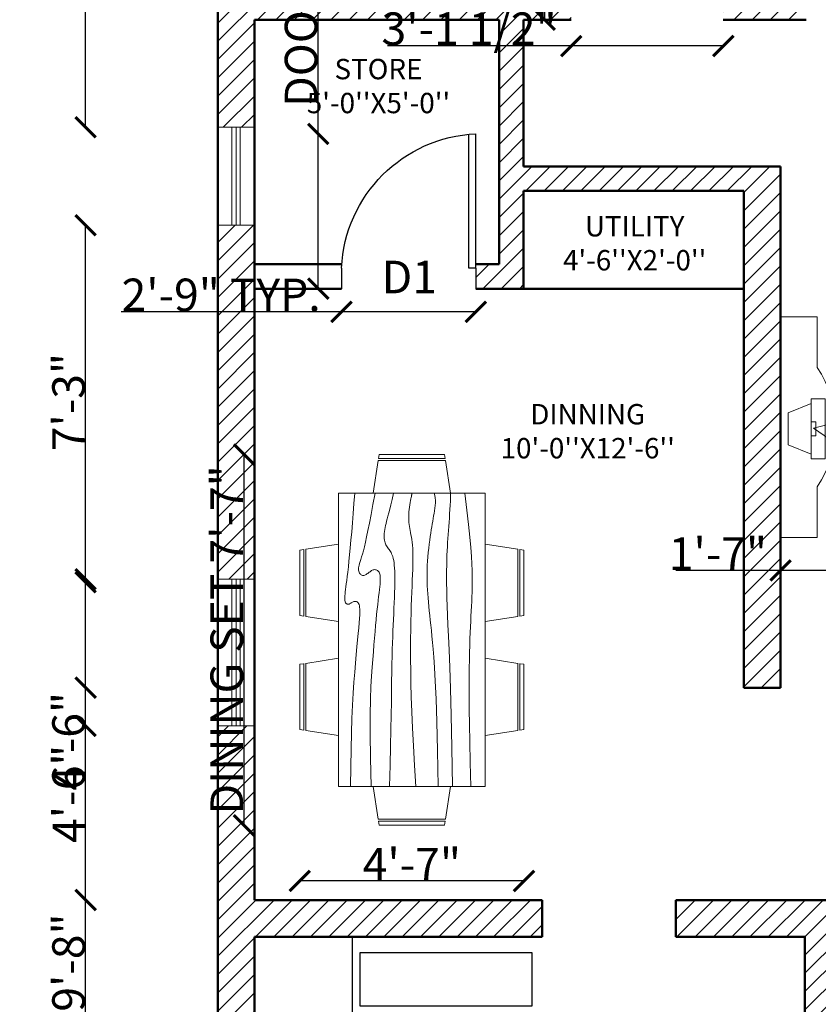
# Model space of a CAD drawing. Units: inches. Extents: x 1385 to 1778, y 1343 to 2100.
# Tile 2 of 6: x 1385 to 1581, y 1579 to 1821. Entities that reach past the tile are written whole.
import ezdxf

# ---------------------------------------------------------------- set-up
doc = ezdxf.new("R2010")
doc.units = ezdxf.units.IN
for name, color, linetype, lineweight in [('A-ANNO-DIMS', 2, 'Continuous', 18), ('A-ANNO-TEXT', 7, 'Continuous', 25), ('A-AREA-IDEN', 7, 'Continuous', 25), ('A-FURN', 8, 'Continuous', 18), ('A-WALL-PATT', 8, 'Continuous', 13), ('Door', 150, 'Continuous', 25), ('Kitchen', 142, 'Continuous', 25), ('Wall', 7, 'Continuous', 50), ('Windows', 140, 'Continuous', 18)]:
    doc.layers.add(name, color=color, linetype=linetype, lineweight=lineweight)
doc.styles.get("Standard").update_dxf_attribs({"font": 'arial.ttf'})
doc.dimstyles.get("Standard").update_dxf_attribs({"dimtxt": 8, "dimasz": 5, "dimexe": 0.18, "dimexo": 0.0625, "dimgap": 0.09, "dimtad": 1, "dimdec": 1, "dimzin": 0, "dimdsep": 46, "dimlunit": 4, "dimtxsty": 'Standard', "dimblk": 'ARCHTICK', "dimcen": 0.09, "dimse1": 1, "dimse2": 1, "dimadec": 0, "dimazin": 0, "dimtfac": 1, "dimtdec": 1, "dimtofl": 0, "dimtmove": 0, "dimatfit": 3, "dimfxl": 1, "dimtolj": 1, "dimtzin": 0, "dimarcsym": 0})

# ---------------------------------------------------------------- blocks, each defined once
blk = doc.blocks.new('AP0B05')
for p, q in [((35, 100), (35, 880)), ((75, 100), (75, 878.9)), ((35, 100), (35, -20)), ((815, 100), (815, -20))]:
    blk.add_line(p, q)
blk.add_lwpolyline([(35, 100), (75, 100)])
blk.add_arc((-2.4, 62.6), 818.3, 2.6212, 87.3788)
blk = doc.blocks.new('Dining Set - 36 x 72 in.')
for p, q in [((-22, 27.5), (-22.1562, 26.50042)), ((-22, 27.5), (-6, 27.5)), ((-5.8437, 26.49966), (-6, 27.5)), ((6, 27.5), (5.8438, 26.50042)), ((6, 27.5), (22, 27.5)), ((22.1563, 26.49966), (22, 27.5)), ((-22.2343, 26.00059), (-23.4847, 17.99762)), ((-22.2304, 26), (-5.7608, 26)), ((-5.8416, 26.5), (-22.1534, 26.5)), ((-4.5152, 17.99762), (-5.7655, 25.99926)), ((5.7657, 26.00059), (4.5153, 17.99762)), ((5.7696, 26), (22.2392, 26)), ((22.1584, 26.5), (5.8466, 26.5)), ((23.4848, 17.99762), (22.2345, 25.99926)), ((36, 18), (-36, 18)), ((-36, 18), (-36, -18)), ((36, -18), (36, 18)), ((-45.5, 8), (-44.5004, 8.15617)), ((-45.5, 8), (-45.5, -8)), ((-44.5, -8.15843), (-44.5, 8.15338)), ((-44.0006, 8.23428), (-35.9976, 9.48474)), ((-44, 8.23041), (-44, -8.23915)), ((44.0006, 8.23428), (35.9976, 9.48474)), ((44, 8.23041), (44, -8.23915)), ((44.5, -8.15843), (44.5, 8.15338)), ((45.5, 8), (44.5005, 8.15617)), ((45.5, 8), (45.5, -8)), ((-44.4997, -8.15631), (-45.5, -8)), ((-35.9976, -9.48476), (-43.9993, -8.2345)), ((35.9976, -9.48476), (43.9993, -8.2345)), ((44.4997, -8.15631), (45.5, -8)), ((-36, -18), (36, -18)), ((-22.2343, -26.0006), (-23.4847, -17.99762)), ((-4.5152, -17.99762), (-5.7655, -25.99928)), ((5.7657, -26.0006), (4.5153, -17.99762)), ((23.4848, -17.99762), (22.2345, -25.99928)), ((-22.2304, -26), (-5.7608, -26)), ((-22, -27.5), (-22.1562, -26.50044)), ((-5.8416, -26.5), (-22.1534, -26.5)), ((-5.8437, -26.49967), (-6, -27.5)), ((5.7696, -26), (22.2392, -26)), ((6, -27.5), (5.8438, -26.50044)), ((22.1584, -26.5), (5.8466, -26.5)), ((22.1563, -26.49967), (22, -27.5)), ((-22, -27.5), (-6, -27.5)), ((6, -27.5), (22, -27.5))]:
    blk.add_line(p, q)
for points in [[(-36, 15), (-31.1772, 14.97754), (-26.8079, 14.91406), (-22.8538, 14.81543), (-19.276, 14.6875), (-16.0362, 14.53613), (-13.0957, 14.36718), (-10.4159, 14.18652), (-7.9583, 14), (-5.6904, 13.81315), (-3.6035, 13.63021), (-1.6954, 13.45508), (0.0365, 13.29166), (1.5945, 13.14388), (2.9811, 13.01562), (4.1988, 12.9108), (5.25, 12.83333), (6.1393, 12.78613), (6.8802, 12.76823), (7.4883, 12.77767), (7.9792, 12.8125), (8.3685, 12.87077), (8.6719, 12.95052), (8.9049, 13.0498), (9.0833, 13.16666), (9.2205, 13.29899), (9.3216, 13.44401), (9.3895, 13.59879), (9.4271, 13.76041), (9.4373, 13.92594), (9.4232, 14.09245), (9.3875, 14.257), (9.3333, 14.41666), (9.2638, 14.56917), (9.1836, 14.71484), (9.0975, 14.85465), (9.0104, 14.98958), (8.9272, 15.1206), (8.8529, 15.2487), (8.7922, 15.37483), (8.75, 15.5), (8.7305, 15.62467), (8.7344, 15.74739), (8.7617, 15.86621), (8.8125, 15.97916), (8.8867, 16.08431), (8.9844, 16.17968), (9.1055, 16.26334), (9.25, 16.33333), (9.4189, 16.38802), (9.6172, 16.42708), (9.8506, 16.45052), (10.125, 16.45833), (10.4463, 16.45052), (10.8203, 16.42708), (11.2529, 16.38802), (11.75, 16.33333), (12.3184, 16.26318), (12.9694, 16.17838), (13.7151, 16.07991), (14.5677, 15.96875), (15.5395, 15.84586), (16.6426, 15.71224), (17.8893, 15.56884), (19.2917, 15.41666), (20.859, 15.25667), (22.5879, 15.08984), (24.4721, 14.91715), (26.5052, 14.73958), (28.6809, 14.5581), (30.9929, 14.3737), (33.4347, 14.18733), (36, 14)], [(-36, 10), (-28.9766, 10.14274), (-23.1725, 10.20442), (-18.4241, 10.19775), (-14.5677, 10.13541), (-11.4399, 10.03011), (-8.877, 9.89453), (-6.7154, 9.74137), (-4.7917, 9.58333), (-2.9698, 9.43082), (-1.2246, 9.28515), (0.4415, 9.14534), (2.026, 9.01041), (3.5266, 8.87939), (4.9408, 8.7513), (6.266, 8.62516), (7.5, 8.5), (8.6411, 8.37549), (9.6914, 8.2539), (10.6538, 8.13818), (11.5312, 8.03125), (12.3267, 7.93603), (13.043, 7.85547), (13.6831, 7.79248), (14.25, 7.75), (14.7471, 7.7303), (15.1797, 7.73307), (15.5537, 7.75732), (15.875, 7.80208), (16.1494, 7.86637), (16.3828, 7.94922), (16.5811, 8.04964), (16.75, 8.16666), (16.8944, 8.29915), (17.0143, 8.44531), (17.1089, 8.60319), (17.1771, 8.77083), (17.218, 8.94629), (17.2305, 9.1276), (17.2137, 9.31282), (17.1667, 9.5), (17.0895, 9.6875), (16.987, 9.875), (16.8649, 10.0625), (16.7292, 10.25), (16.5856, 10.4375), (16.4401, 10.625), (16.2985, 10.8125), (16.1667, 11), (16.05, 11.18733), (15.9518, 11.3737), (15.8752, 11.5581), (15.8229, 11.73958), (15.798, 11.91715), (15.8034, 12.08984), (15.842, 12.25667), (15.9167, 12.41666), (16.0295, 12.56836), (16.1784, 12.70833), (16.3605, 12.83268), (16.5729, 12.9375), (16.8127, 13.01888), (17.0768, 13.07291), (17.3625, 13.0957), (17.6667, 13.08333), (17.9894, 13.03312), (18.3418, 12.94726), (18.7382, 12.82918), (19.1927, 12.68229), (19.7195, 12.51001), (20.3327, 12.31575), (21.0465, 12.10294), (21.875, 11.875), (22.8357, 11.63354), (23.959, 11.37304), (25.2786, 11.08618), (26.8282, 10.76562), (28.6414, 10.40405), (30.752, 9.99414), (33.1936, 9.52856), (36, 9)], [(-36, 5.5), (-30.7157, 5.3348), (-26.069, 5.20963), (-21.9946, 5.11767), (-18.4271, 5.05208), (-15.3009, 5.00602), (-12.5508, 4.97265), (-10.1112, 4.94515), (-7.9167, 4.91666), (-5.909, 4.88167), (-4.0586, 4.83984), (-2.3429, 4.79215), (-0.7396, 4.73958), (0.7739, 4.6831), (2.22, 4.6237), (3.6213, 4.56233), (5, 4.5), (6.373, 4.43782), (7.7344, 4.3776), (9.0723, 4.32129), (10.375, 4.27083), (11.6309, 4.22819), (12.8281, 4.19531), (13.9551, 4.17415), (15, 4.16666), (15.954, 4.17448), (16.819, 4.19791), (17.6001, 4.23698), (18.3021, 4.29166), (18.9299, 4.36198), (19.4883, 4.44791), (19.9823, 4.54948), (20.4167, 4.66666), (20.7969, 4.79899), (21.1302, 4.94401), (21.4245, 5.09879), (21.6875, 5.26041), (21.9271, 5.42594), (22.1511, 5.59245), (22.3672, 5.757), (22.5834, 5.91666), (22.8065, 6.06868), (23.0404, 6.21093), (23.2879, 6.34147), (23.5521, 6.45833), (23.8358, 6.55957), (24.142, 6.64323), (24.4735, 6.70735), (24.8334, 6.75), (25.2235, 6.76969), (25.642, 6.76692), (26.0858, 6.74267), (26.5521, 6.69791), (27.0379, 6.63362), (27.5404, 6.55078), (28.0565, 6.45036), (28.5834, 6.33333), (29.1242, 6.19987), (29.7071, 6.04687), (30.3661, 5.87044), (31.1354, 5.66666), (32.0493, 5.43164), (33.142, 5.16146), (34.4475, 4.85221), (36, 4.5)], [(-36, -1), (-30.7915, -0.6591), (-26.0195, -0.38216), (-21.6519, -0.16284), (-17.6563, 0.00521), (-14.0005, 0.12833), (-10.6523, 0.21289), (-7.5796, 0.26522), (-4.75, 0.29166), (-2.134, 0.29793), (0.2878, 0.28711), (2.5317, 0.26163), (4.6146, 0.22396), (6.5529, 0.17651), (8.3633, 0.12174), (10.0623, 0.06209), (11.6667, 0), (13.1899, -0.06201), (14.6341, -0.1211), (15.9982, -0.17432), (17.2813, -0.21875), (18.4823, -0.25147), (19.6003, -0.26953), (20.6343, -0.27002), (21.5834, -0.25), (22.4481, -0.20768), (23.2357, -0.14584), (23.9549, -0.06836), (24.6146, 0.02083), (25.2235, 0.11784), (25.7904, 0.21875), (26.3241, 0.31966), (26.8334, 0.41666), (27.3265, 0.50618), (27.8099, 0.58593), (28.2894, 0.65397), (28.7709, 0.70833), (29.2601, 0.74707), (29.763, 0.76823), (30.2855, 0.76985), (30.8334, 0.75), (31.4088, 0.70784), (31.9994, 0.64713), (32.589, 0.57275), (33.1615, 0.48958), (33.7008, 0.4025), (34.1908, 0.3164), (34.6153, 0.23616), (34.9584, 0.16666), (35.2099, 0.11165), (35.3848, 0.07031), (35.504, 0.04069), (35.5886, 0.02083), (35.6594, 0.00879), (35.7377, 0.0026), (35.8442, 0.00032), (36, 0)], [(-36, -6.5), (-27.1843, -6.31267), (-20.084, -6.1263), (-14.469, -5.9419), (-10.1094, -5.76042), (-6.7752, -5.58285), (-4.2363, -5.41016), (-2.2629, -5.24333), (-0.625, -5.08334), (0.8708, -4.93099), (2.2715, -4.78646), (3.5872, -4.64974), (4.8281, -4.52084), (6.0046, -4.39974), (7.127, -4.28646), (8.2053, -4.18099), (9.25, -4.08334), (10.2705, -3.99382), (11.2734, -3.91407), (12.2647, -3.84603), (13.25, -3.79167), (14.2354, -3.75293), (15.2266, -3.73177), (16.2295, -3.73015), (17.25, -3.75), (18.2912, -3.79248), (19.3451, -3.85547), (20.4009, -3.93604), (21.4479, -4.03125), (22.4754, -4.13819), (23.4727, -4.25391), (24.4289, -4.37549), (25.3334, -4.5), (26.1785, -4.62492), (26.9694, -4.74935), (27.7145, -4.87281), (28.4219, -4.99479), (29.1, -5.11483), (29.7572, -5.23242), (30.4016, -5.34709), (31.0417, -5.45834), (31.6837, -5.56437), (32.3262, -5.65821), (32.9658, -5.73153), (33.599, -5.77604), (34.2224, -5.78345), (34.8327, -5.74545), (35.4264, -5.65373), (36, -5.5)], [(-36, -10), (-26.4022, -9.81299), (-18.4675, -9.62891), (-11.9839, -9.45069), (-6.7396, -9.28125), (-2.5226, -9.12354), (0.8789, -8.98047), (3.6769, -8.85498), (6.0833, -8.75), (8.2767, -8.66765), (10.3021, -8.60677), (12.1712, -8.56543), (13.8958, -8.54167), (15.4876, -8.53353), (16.9583, -8.53907), (18.3197, -8.55632), (19.5834, -8.58334), (20.7616, -8.61841), (21.8685, -8.66081), (22.9188, -8.71004), (23.9271, -8.76563), (24.9081, -8.82707), (25.8763, -8.89388), (26.8465, -8.96558), (27.8334, -9.04167), (28.8474, -9.12118), (29.8828, -9.20117), (30.93, -9.27824), (31.9792, -9.34896), (33.0205, -9.40991), (34.0443, -9.45768), (35.0407, -9.48885), (36, -9.5)], [(-36, -14.5), (-30.0881, -14.33513), (-25.0332, -14.21224), (-20.7312, -14.12647), (-17.0781, -14.07292), (-13.97, -14.04671), (-11.3027, -14.04297), (-8.9724, -14.05681), (-6.875, -14.08334), (-4.9224, -14.11833), (-3.0905, -14.16016), (-1.3709, -14.20785), (0.2448, -14.26042), (1.7647, -14.3169), (3.1973, -14.3763), (4.5507, -14.43767), (5.8333, -14.5), (7.0554, -14.5621), (8.235, -14.62175), (9.3922, -14.67652), (10.5469, -14.72396), (11.7192, -14.76164), (12.929, -14.78711), (14.1965, -14.79794), (15.5417, -14.79167), (16.9933, -14.76424), (18.6152, -14.70508), (20.4804, -14.60197), (22.6615, -14.44271), (25.2312, -14.21509), (28.2624, -13.9069), (31.8277, -13.50594), (36, -13)]]:
    blk.add_lwpolyline(points)
blk = doc.blocks.new('banghe81')
for p, q in [((-500, 3000), (0, 3000)), ((-500, 2312), (-500, 3000)), ((0, 3000), (0, 0)), ((-607, 1930), (-419, 1930)), ((-607, 1117), (-607, 1930)), ((-419, 1930), (-419, 1117)), ((-925, 1843), (-450, 1517)), ((-107, 1742), (-419, 1867)), ((-107, 1305), (-107, 1742)), ((-482, 1617), (-482, 1430)), ((-419, 1617), (-482, 1617)), ((-450, 1517), (-1057, 1361)), ((-482, 1430), (-419, 1430)), ((-419, 1180), (-107, 1305)), ((-419, 1117), (-607, 1117)), ((-500, 0), (-500, 688)), ((0, 0), (-500, 0)), ((-500, 0), (-500, 0))]:
    blk.add_line(p, q)
blk.add_arc((695, 1500), 1445, 145.7945, 214.2055)
blk = doc.blocks.new('WINDOW-GLAZING-36IN')
for p, q in [((0, 0), (0, 36)), ((1, 0), (1, 36)), ((2, 0), (2, 36))]:
    blk.add_line(p, q)
blk = doc.blocks.new('WINDOW-GLAZING-24IN')
for p, q in [((0, 2), (24, 2)), ((0, 1), (24, 1)), ((0, 0), (24, 0))]:
    blk.add_line(p, q)
blk = doc.blocks.new('_ArchTick')
at = {"color": 0, "linetype": 'ByBlock', "const_width": 0.15}
blk.add_lwpolyline([(-0.5, -0.5), (0.5, 0.5)], dxfattribs=at)
blk = doc.blocks.new('*D19')
at = {"layer": 'A-ANNO-DIMS', "color": 0, "lineweight": -2, "transparency": 16777216}
for p, q in [((1458.44, 1792.72), (1458.44, 1882.9)), ((1458.44, 1754.73), (1458.44, 1792.72))]:
    blk.add_line(p, q, dxfattribs=at)
at = {"layer": 'Defpoints', "color": 0, "transparency": 16777216}
for p in [(1458.44, 1792.72), (1464.14, 1792.72), (1464.14, 1754.73)]:
    blk.add_point(p, dxfattribs=at)
at = {"layer": 'A-ANNO-DIMS', "color": 0, "lineweight": -2, "transparency": 16777216, "xscale": 5, "yscale": 5, "zscale": 5}
for p, rotation in [((1458.44, 1792.72), 90), ((1458.44, 1754.73), 270)]:
    blk.add_blockref('_ArchTick', p, dxfattribs=dict(at, rotation=rotation))
at = {"layer": 'A-ANNO-DIMS', "color": 0, "transparency": 16777216, "insert": (1454.21, 1840.31), "char_height": 8, "attachment_point": 5, "rotation": 90}
blk.add_mtext('\\A1;DOOR 3\'-2" TYP.', dxfattribs=at)
blk = doc.blocks.new('*D20')
at = {"layer": 'A-ANNO-DIMS', "color": 0, "lineweight": -2, "transparency": 16777216}
for p, q in [((1464.14, 1749.04), (1410.06, 1749.04)), ((1497.07, 1749.04), (1464.14, 1749.04))]:
    blk.add_line(p, q, dxfattribs=at)
at = {"layer": 'Defpoints', "color": 0, "transparency": 16777216}
for p in [(1464.14, 1754.73), (1497.07, 1754.73), (1464.14, 1749.04)]:
    blk.add_point(p, dxfattribs=at)
at = {"layer": 'A-ANNO-DIMS', "color": 0, "lineweight": -2, "transparency": 16777216, "xscale": 5, "yscale": 5, "zscale": 5, "rotation": 180}
blk.add_blockref('_ArchTick', (1464.14, 1749.04), dxfattribs=at)
at = {"layer": 'A-ANNO-DIMS', "color": 0, "lineweight": -2, "transparency": 16777216, "xscale": 5, "yscale": 5, "zscale": 5}
blk.add_blockref('_ArchTick', (1497.07, 1749.04), dxfattribs=at)
at = {"layer": 'A-ANNO-DIMS', "color": 0, "transparency": 16777216, "insert": (1434.6, 1753.21), "char_height": 8, "attachment_point": 5}
blk.add_mtext('\\A1;2\'-9" TYP.', dxfattribs=at)
blk = doc.blocks.new('*D21')
at = {"layer": 'A-ANNO-DIMS', "color": 0, "lineweight": -2, "transparency": 16777216}
for p, q in [((1513.99, 1863.79), (1513.99, 1926.47)), ((1513.99, 1820.73), (1513.99, 1863.79))]:
    blk.add_line(p, q, dxfattribs=at)
at = {"layer": 'Defpoints', "color": 0, "transparency": 16777216}
for p in [(1513.99, 1863.79), (1520.45, 1863.79), (1520.45, 1820.73)]:
    blk.add_point(p, dxfattribs=at)
at = {"layer": 'A-ANNO-DIMS', "color": 0, "lineweight": -2, "transparency": 16777216, "xscale": 5, "yscale": 5, "zscale": 5}
for p, rotation in [((1513.99, 1863.79), 90), ((1513.99, 1820.73), 270)]:
    blk.add_blockref('_ArchTick', p, dxfattribs=dict(at, rotation=rotation))
at = {"layer": 'A-ANNO-DIMS', "color": 0, "transparency": 16777216, "insert": (1509.76, 1897.63), "char_height": 8, "attachment_point": 5, "rotation": 90}
blk.add_mtext('\\A1;DOOR 3\'-7"', dxfattribs=at)
blk = doc.blocks.new('*D22')
at = {"layer": 'A-ANNO-DIMS', "color": 0, "lineweight": -2, "transparency": 16777216}
for p, q in [((1520.45, 1814.28), (1475.37, 1814.28)), ((1557.76, 1814.28), (1520.45, 1814.28))]:
    blk.add_line(p, q, dxfattribs=at)
at = {"layer": 'Defpoints', "color": 0, "transparency": 16777216}
for p in [(1520.45, 1820.73), (1557.76, 1820.73), (1520.45, 1814.28)]:
    blk.add_point(p, dxfattribs=at)
at = {"layer": 'A-ANNO-DIMS', "color": 0, "lineweight": -2, "transparency": 16777216, "xscale": 5, "yscale": 5, "zscale": 5, "rotation": 180}
blk.add_blockref('_ArchTick', (1520.45, 1814.28), dxfattribs=at)
at = {"layer": 'A-ANNO-DIMS', "color": 0, "lineweight": -2, "transparency": 16777216, "xscale": 5, "yscale": 5, "zscale": 5}
blk.add_blockref('_ArchTick', (1557.76, 1814.28), dxfattribs=at)
at = {"layer": 'A-ANNO-DIMS', "color": 0, "transparency": 16777216, "insert": (1495.41, 1818.51), "char_height": 8, "attachment_point": 5}
blk.add_mtext('\\A1;3\'-1 1/2"', dxfattribs=at)
blk = doc.blocks.new('*D45')
at = {"layer": 'A-ANNO-DIMS', "color": 0, "lineweight": -2, "transparency": 16777216}
blk.add_line((1440.22, 1623.07), (1440.22, 1714.07), dxfattribs=at)
at = {"layer": 'Defpoints', "color": 0, "transparency": 16777216}
for p in [(1440.22, 1714.07), (1453.87, 1714.07), (1453.87, 1623.07)]:
    blk.add_point(p, dxfattribs=at)
at = {"layer": 'A-ANNO-DIMS', "color": 0, "lineweight": -2, "transparency": 16777216, "xscale": 5, "yscale": 5, "zscale": 5}
for p, rotation in [((1440.22, 1714.07), 90), ((1440.22, 1623.07), 270)]:
    blk.add_blockref('_ArchTick', p, dxfattribs=dict(at, rotation=rotation))
at = {"layer": 'A-ANNO-DIMS', "color": 0, "transparency": 16777216, "insert": (1435.99, 1668.57), "char_height": 8, "attachment_point": 5, "rotation": 90}
blk.add_mtext('\\A1;DINING SET 7\'-7"', dxfattribs=at)
blk = doc.blocks.new('*D46')
at = {"layer": 'A-ANNO-DIMS', "color": 0, "lineweight": -2, "transparency": 16777216}
blk.add_line((1508.87, 1609.42), (1453.87, 1609.42), dxfattribs=at)
at = {"layer": 'Defpoints', "color": 0, "transparency": 16777216}
for p in [(1453.87, 1623.07), (1508.87, 1623.07), (1453.87, 1609.42)]:
    blk.add_point(p, dxfattribs=at)
at = {"layer": 'A-ANNO-DIMS', "color": 0, "lineweight": -2, "transparency": 16777216, "xscale": 5, "yscale": 5, "zscale": 5, "rotation": 180}
blk.add_blockref('_ArchTick', (1453.87, 1609.42), dxfattribs=at)
at = {"layer": 'A-ANNO-DIMS', "color": 0, "lineweight": -2, "transparency": 16777216, "xscale": 5, "yscale": 5, "zscale": 5}
blk.add_blockref('_ArchTick', (1508.87, 1609.42), dxfattribs=at)
at = {"layer": 'A-ANNO-DIMS', "color": 0, "transparency": 16777216, "insert": (1481.37, 1613.51), "char_height": 8, "attachment_point": 5}
blk.add_mtext('\\A1;4\'-7"', dxfattribs=at)
blk = doc.blocks.new('*D47')
at = {"layer": 'A-ANNO-DIMS', "color": 0, "lineweight": -2, "transparency": 16777216}
for p, q in [((1598.95, 1747.83), (1598.95, 1693.73)), ((1598.95, 1693.73), (1598.95, 1620.51))]:
    blk.add_line(p, q, dxfattribs=at)
at = {"layer": 'Defpoints', "color": 0, "transparency": 16777216}
for p in [(1590.84, 1747.83), (1590.84, 1693.73), (1598.95, 1693.73)]:
    blk.add_point(p, dxfattribs=at)
at = {"layer": 'A-ANNO-DIMS', "color": 0, "lineweight": -2, "transparency": 16777216, "xscale": 5, "yscale": 5, "zscale": 5}
for p, rotation in [((1598.95, 1747.83), 90), ((1598.95, 1693.73), 270)]:
    blk.add_blockref('_ArchTick', p, dxfattribs=dict(at, rotation=rotation))
at = {"layer": 'A-ANNO-DIMS', "color": 0, "transparency": 16777216, "insert": (1594.78, 1654.62), "char_height": 8, "attachment_point": 5, "rotation": 90}
blk.add_mtext('\\A1;TV UNIT 4\'-6"', dxfattribs=at)
blk = doc.blocks.new('*D48')
at = {"layer": 'A-ANNO-DIMS', "color": 0, "lineweight": -2, "transparency": 16777216}
for p, q in [((1571.77, 1685.61), (1546.08, 1685.61)), ((1590.84, 1685.61), (1571.77, 1685.61))]:
    blk.add_line(p, q, dxfattribs=at)
at = {"layer": 'Defpoints', "color": 0, "transparency": 16777216}
for p in [(1571.77, 1693.73), (1590.84, 1693.73), (1571.77, 1685.61)]:
    blk.add_point(p, dxfattribs=at)
at = {"layer": 'A-ANNO-DIMS', "color": 0, "lineweight": -2, "transparency": 16777216, "xscale": 5, "yscale": 5, "zscale": 5, "rotation": 180}
blk.add_blockref('_ArchTick', (1571.77, 1685.61), dxfattribs=at)
at = {"layer": 'A-ANNO-DIMS', "color": 0, "lineweight": -2, "transparency": 16777216, "xscale": 5, "yscale": 5, "zscale": 5}
blk.add_blockref('_ArchTick', (1590.84, 1685.61), dxfattribs=at)
at = {"layer": 'A-ANNO-DIMS', "color": 0, "transparency": 16777216, "insert": (1556.43, 1689.72), "char_height": 8, "attachment_point": 5}
blk.add_mtext('\\A1;1\'-7"', dxfattribs=at)
blk = doc.blocks.new('*D55')
at = {"layer": 'A-ANNO-DIMS', "color": 0, "lineweight": -2, "transparency": 16777216}
blk.add_line((1401.37, 1604.73), (1401.37, 1682.73), dxfattribs=at)
at = {"layer": 'Defpoints', "color": 0, "transparency": 16777216}
for p in [(1401.37, 1682.73), (1718.77, 1682.73), (1718.77, 1604.73)]:
    blk.add_point(p, dxfattribs=at)
at = {"layer": 'A-ANNO-DIMS', "color": 0, "lineweight": -2, "transparency": 16777216, "xscale": 5, "yscale": 5, "zscale": 5}
for p, rotation in [((1401.37, 1682.73), 90), ((1401.37, 1604.73), 270)]:
    blk.add_blockref('_ArchTick', p, dxfattribs=dict(at, rotation=rotation))
at = {"layer": 'A-ANNO-DIMS', "color": 0, "transparency": 16777216, "insert": (1397.19, 1643.73), "char_height": 8, "attachment_point": 5, "rotation": 90}
blk.add_mtext('\\A1;6\'-6"', dxfattribs=at)
blk = doc.blocks.new('*D57')
at = {"layer": 'A-ANNO-DIMS', "color": 0, "lineweight": -2, "transparency": 16777216}
for p, q in [((1401.37, 1840.6), (1401.37, 1891.9)), ((1401.37, 1794.33), (1401.37, 1840.6))]:
    blk.add_line(p, q, dxfattribs=at)
at = {"layer": 'Defpoints', "color": 0, "transparency": 16777216}
for p in [(1401.37, 1840.6), (1433.77, 1840.6), (1433.77, 1794.33)]:
    blk.add_point(p, dxfattribs=at)
at = {"layer": 'A-ANNO-DIMS', "color": 0, "lineweight": -2, "transparency": 16777216, "xscale": 5, "yscale": 5, "zscale": 5}
for p, rotation in [((1401.37, 1840.6), 90), ((1401.37, 1794.33), 270)]:
    blk.add_blockref('_ArchTick', p, dxfattribs=dict(at, rotation=rotation))
at = {"layer": 'A-ANNO-DIMS', "color": 0, "transparency": 16777216, "insert": (1397.14, 1868.75), "char_height": 8, "attachment_point": 5, "rotation": 90}
blk.add_mtext('\\A1;3\'-10 1/2"', dxfattribs=at)
blk = doc.blocks.new('*D58')
at = {"layer": 'A-ANNO-DIMS', "color": 0, "lineweight": -2, "transparency": 16777216}
blk.add_line((1401.37, 1683.46), (1401.37, 1770.33), dxfattribs=at)
at = {"layer": 'Defpoints', "color": 0, "transparency": 16777216}
for p in [(1401.37, 1770.33), (1433.77, 1770.33), (1433.77, 1683.46)]:
    blk.add_point(p, dxfattribs=at)
at = {"layer": 'A-ANNO-DIMS', "color": 0, "lineweight": -2, "transparency": 16777216, "xscale": 5, "yscale": 5, "zscale": 5}
for p, rotation in [((1401.37, 1770.33), 90), ((1401.37, 1683.46), 270)]:
    blk.add_blockref('_ArchTick', p, dxfattribs=dict(at, rotation=rotation))
at = {"layer": 'A-ANNO-DIMS', "color": 0, "transparency": 16777216, "insert": (1397.19, 1726.9), "char_height": 8, "attachment_point": 5, "rotation": 90}
blk.add_mtext('\\A1;7\'-3"', dxfattribs=at)
blk = doc.blocks.new('*D59')
at = {"layer": 'A-ANNO-DIMS', "color": 0, "lineweight": -2, "transparency": 16777216}
blk.add_line((1401.37, 1531.33), (1401.37, 1647.46), dxfattribs=at)
at = {"layer": 'Defpoints', "color": 0, "transparency": 16777216}
for p in [(1401.37, 1647.46), (1433.77, 1647.46), (1433.77, 1531.33)]:
    blk.add_point(p, dxfattribs=at)
at = {"layer": 'A-ANNO-DIMS', "color": 0, "lineweight": -2, "transparency": 16777216, "xscale": 5, "yscale": 5, "zscale": 5}
for p, rotation in [((1401.37, 1647.46), 90), ((1401.37, 1531.33), 270)]:
    blk.add_blockref('_ArchTick', p, dxfattribs=dict(at, rotation=rotation))
at = {"layer": 'A-ANNO-DIMS', "color": 0, "transparency": 16777216, "insert": (1397.19, 1589.39), "char_height": 8, "attachment_point": 5, "rotation": 90}
blk.add_mtext('\\A1;9\'-8"', dxfattribs=at)
blk = doc.blocks.new('*D62')
at = {"layer": 'A-ANNO-DIMS', "color": 0, "lineweight": -2, "transparency": 16777216}
for p, q in [((1442.77, 2063.14), (1475.11, 2063.14)), ((1475.11, 2063.14), (1520.34, 2063.14))]:
    blk.add_line(p, q, dxfattribs=at)
at = {"layer": 'Defpoints', "color": 0, "transparency": 16777216}
for p in [(1475.11, 2063.14), (1442.77, 1391.73), (1475.11, 1391.73)]:
    blk.add_point(p, dxfattribs=at)
at = {"layer": 'A-ANNO-DIMS', "color": 0, "lineweight": -2, "transparency": 16777216, "xscale": 5, "yscale": 5, "zscale": 5, "rotation": 180}
blk.add_blockref('_ArchTick', (1442.77, 2063.14), dxfattribs=at)
at = {"layer": 'A-ANNO-DIMS', "color": 0, "lineweight": -2, "transparency": 16777216, "xscale": 5, "yscale": 5, "zscale": 5}
blk.add_blockref('_ArchTick', (1475.11, 2063.14), dxfattribs=at)
at = {"layer": 'A-ANNO-DIMS', "color": 0, "transparency": 16777216, "insert": (1500.22, 2067.37), "char_height": 8, "attachment_point": 5}
blk.add_mtext('\\A1;2\'-8 1/2"', dxfattribs=at)
blk = doc.blocks.new('*D63')
at = {"layer": 'A-ANNO-DIMS', "color": 0, "lineweight": -2, "transparency": 16777216}
for p, q in [((1475.11, 2063.14), (1485.11, 2063.14)), ((1485.11, 2063.14), (1517.77, 2063.14))]:
    blk.add_line(p, q, dxfattribs=at)
at = {"layer": 'Defpoints', "color": 0, "transparency": 16777216}
for p in [(1485.11, 2063.14), (1475.11, 1391.73), (1485.11, 1391.73)]:
    blk.add_point(p, dxfattribs=at)
at = {"layer": 'A-ANNO-DIMS', "color": 0, "lineweight": -2, "transparency": 16777216, "xscale": 5, "yscale": 5, "zscale": 5, "rotation": 180}
blk.add_blockref('_ArchTick', (1475.11, 2063.14), dxfattribs=at)
at = {"layer": 'A-ANNO-DIMS', "color": 0, "lineweight": -2, "transparency": 16777216, "xscale": 5, "yscale": 5, "zscale": 5}
blk.add_blockref('_ArchTick', (1485.11, 2063.14), dxfattribs=at)
at = {"layer": 'A-ANNO-DIMS', "color": 0, "transparency": 16777216, "insert": (1503.94, 2067.31), "char_height": 8, "attachment_point": 5}
blk.add_mtext('\\A1;0\'-10"', dxfattribs=at)
blk = doc.blocks.new('*D65')
at = {"layer": 'A-ANNO-DIMS', "color": 0, "lineweight": -2, "transparency": 16777216}
blk.add_line((1442.77, 1350.33), (1466.77, 1350.33), dxfattribs=at)
at = {"layer": 'Defpoints', "color": 0, "transparency": 16777216}
for p in [(1442.77, 1595.73), (1466.77, 1595.73), (1466.77, 1350.33)]:
    blk.add_point(p, dxfattribs=at)
at = {"layer": 'A-ANNO-DIMS', "color": 0, "lineweight": -2, "transparency": 16777216, "xscale": 5, "yscale": 5, "zscale": 5, "rotation": 180}
blk.add_blockref('_ArchTick', (1442.77, 1350.33), dxfattribs=at)
at = {"layer": 'A-ANNO-DIMS', "color": 0, "lineweight": -2, "transparency": 16777216, "xscale": 5, "yscale": 5, "zscale": 5}
blk.add_blockref('_ArchTick', (1466.77, 1350.33), dxfattribs=at)
at = {"layer": 'A-ANNO-DIMS', "color": 0, "transparency": 16777216, "insert": (1454.77, 1354.5), "char_height": 8, "attachment_point": 5}
blk.add_mtext('\\A1;2\'-0"', dxfattribs=at)
blk = doc.blocks.new('*D66')
at = {"layer": 'A-ANNO-DIMS', "color": 0, "lineweight": -2, "transparency": 16777216}
blk.add_line((1442.77, 2063.14), (1513.34, 2063.14), dxfattribs=at)
at = {"layer": 'Defpoints', "color": 0, "transparency": 16777216}
for p in [(1513.34, 2063.14), (1442.77, 1595.73), (1513.34, 1595.73)]:
    blk.add_point(p, dxfattribs=at)
at = {"layer": 'A-ANNO-DIMS', "color": 0, "lineweight": -2, "transparency": 16777216, "xscale": 5, "yscale": 5, "zscale": 5, "rotation": 180}
blk.add_blockref('_ArchTick', (1442.77, 2063.14), dxfattribs=at)
at = {"layer": 'A-ANNO-DIMS', "color": 0, "lineweight": -2, "transparency": 16777216, "xscale": 5, "yscale": 5, "zscale": 5}
blk.add_blockref('_ArchTick', (1513.34, 2063.14), dxfattribs=at)
at = {"layer": 'A-ANNO-DIMS', "color": 0, "transparency": 16777216, "insert": (1478.05, 2067.37), "char_height": 8, "attachment_point": 5}
blk.add_mtext('\\A1;5\'-10 1/2"', dxfattribs=at)
blk = doc.blocks.new('*D67')
at = {"layer": 'A-ANNO-DIMS', "color": 0, "lineweight": -2, "transparency": 16777216}
for p, q in [((1513.34, 2063.14), (1546.08, 2063.14)), ((1546.08, 2063.14), (1591.31, 2063.14))]:
    blk.add_line(p, q, dxfattribs=at)
at = {"layer": 'Defpoints', "color": 0, "transparency": 16777216}
for p in [(1546.08, 2063.14), (1513.34, 1595.73), (1546.08, 1595.73)]:
    blk.add_point(p, dxfattribs=at)
at = {"layer": 'A-ANNO-DIMS', "color": 0, "lineweight": -2, "transparency": 16777216, "xscale": 5, "yscale": 5, "zscale": 5, "rotation": 180}
blk.add_blockref('_ArchTick', (1513.34, 2063.14), dxfattribs=at)
at = {"layer": 'A-ANNO-DIMS', "color": 0, "lineweight": -2, "transparency": 16777216, "xscale": 5, "yscale": 5, "zscale": 5}
blk.add_blockref('_ArchTick', (1546.08, 2063.14), dxfattribs=at)
at = {"layer": 'A-ANNO-DIMS', "color": 0, "transparency": 16777216, "insert": (1571.19, 2067.37), "char_height": 8, "attachment_point": 5}
blk.add_mtext('\\A1;2\'-8 1/2"', dxfattribs=at)
blk = doc.blocks.new('*D73')
at = {"layer": 'A-ANNO-DIMS', "color": 0, "lineweight": -2, "transparency": 16777216}
blk.add_line((1468.71, 2063.14), (1494.47, 2063.14), dxfattribs=at)
at = {"layer": 'Defpoints', "color": 0, "transparency": 16777216}
for p in [(1494.47, 2063.14), (1468.71, 1493.49), (1494.47, 1493.49)]:
    blk.add_point(p, dxfattribs=at)
at = {"layer": 'A-ANNO-DIMS', "color": 0, "lineweight": -2, "transparency": 16777216, "xscale": 5, "yscale": 5, "zscale": 5, "rotation": 180}
blk.add_blockref('_ArchTick', (1468.71, 2063.14), dxfattribs=at)
at = {"layer": 'A-ANNO-DIMS', "color": 0, "lineweight": -2, "transparency": 16777216, "xscale": 5, "yscale": 5, "zscale": 5}
blk.add_blockref('_ArchTick', (1494.47, 2063.14), dxfattribs=at)
at = {"layer": 'A-ANNO-DIMS', "color": 0, "transparency": 16777216, "insert": (1481.59, 2067.25), "char_height": 8, "attachment_point": 5}
blk.add_mtext('\\A1;2\'-2"', dxfattribs=at)
blk = doc.blocks.new('*D77')
at = {"layer": 'A-ANNO-DIMS', "color": 0, "lineweight": -2, "transparency": 16777216}
for p, q in [((1497.07, 2063.14), (1502.77, 2063.14)), ((1502.77, 2063.14), (1547.86, 2063.14))]:
    blk.add_line(p, q, dxfattribs=at)
at = {"layer": 'Defpoints', "color": 0, "transparency": 16777216}
for p in [(1502.77, 2063.14), (1497.07, 1760.73), (1502.77, 1760.73)]:
    blk.add_point(p, dxfattribs=at)
at = {"layer": 'A-ANNO-DIMS', "color": 0, "lineweight": -2, "transparency": 16777216, "xscale": 5, "yscale": 5, "zscale": 5, "rotation": 180}
blk.add_blockref('_ArchTick', (1497.07, 2063.14), dxfattribs=at)
at = {"layer": 'A-ANNO-DIMS', "color": 0, "lineweight": -2, "transparency": 16777216, "xscale": 5, "yscale": 5, "zscale": 5}
blk.add_blockref('_ArchTick', (1502.77, 2063.14), dxfattribs=at)
at = {"layer": 'A-ANNO-DIMS', "color": 0, "transparency": 16777216, "insert": (1527.82, 2067.37), "char_height": 8, "attachment_point": 5}
blk.add_mtext('\\A1;0\'-5 1/2"', dxfattribs=at)
blk = doc.blocks.new('*D78')
at = {"layer": 'A-ANNO-DIMS', "color": 0, "lineweight": -2, "transparency": 16777216}
blk.add_line((1401.37, 1604.73), (1401.37, 1656.82), dxfattribs=at)
at = {"layer": 'Defpoints', "color": 0, "transparency": 16777216}
for p in [(1401.37, 1656.82), (1562.77, 1656.82), (1546.08, 1604.73)]:
    blk.add_point(p, dxfattribs=at)
at = {"layer": 'A-ANNO-DIMS', "color": 0, "lineweight": -2, "transparency": 16777216, "xscale": 5, "yscale": 5, "zscale": 5}
for p, rotation in [((1401.37, 1656.82), 90), ((1401.37, 1604.73), 270)]:
    blk.add_blockref('_ArchTick', p, dxfattribs=dict(at, rotation=rotation))
at = {"layer": 'A-ANNO-DIMS', "color": 0, "transparency": 16777216, "insert": (1397.28, 1630.78), "char_height": 8, "attachment_point": 5, "rotation": 90}
blk.add_mtext('\\A1;4\'-4"', dxfattribs=at)
blk = doc.blocks.new('*D79')
at = {"layer": 'A-ANNO-DIMS', "color": 0, "lineweight": -2, "transparency": 16777216}
blk.add_line((1760.18, 1784.73), (1760.18, 1820.73), dxfattribs=at)
at = {"layer": 'Defpoints', "color": 0, "transparency": 16777216}
for p in [(1508.77, 1820.73), (1760.18, 1820.73), (1508.77, 1784.73)]:
    blk.add_point(p, dxfattribs=at)
at = {"layer": 'A-ANNO-DIMS', "color": 0, "lineweight": -2, "transparency": 16777216, "xscale": 5, "yscale": 5, "zscale": 5}
for p, rotation in [((1760.18, 1820.73), 90), ((1760.18, 1784.73), 270)]:
    blk.add_blockref('_ArchTick', p, dxfattribs=dict(at, rotation=rotation))
at = {"layer": 'A-ANNO-DIMS', "color": 0, "transparency": 16777216, "insert": (1756, 1802.73), "char_height": 8, "attachment_point": 5, "rotation": 90}
blk.add_mtext('\\A1;3\'-0"', dxfattribs=at)
blk = doc.blocks.new('*D81')
at = {"layer": 'A-ANNO-DIMS', "color": 0, "lineweight": -2, "transparency": 16777216}
for p, q in [((1760.18, 1591.85), (1760.18, 1617.54)), ((1760.18, 1578.65), (1760.18, 1591.85))]:
    blk.add_line(p, q, dxfattribs=at)
at = {"layer": 'Defpoints', "color": 0, "transparency": 16777216}
for p in [(1510.83, 1591.85), (1760.18, 1591.85), (1510.83, 1578.65)]:
    blk.add_point(p, dxfattribs=at)
at = {"layer": 'A-ANNO-DIMS', "color": 0, "lineweight": -2, "transparency": 16777216, "xscale": 5, "yscale": 5, "zscale": 5}
for p, rotation in [((1760.18, 1591.85), 90), ((1760.18, 1578.65), 270)]:
    blk.add_blockref('_ArchTick', p, dxfattribs=dict(at, rotation=rotation))
at = {"layer": 'A-ANNO-DIMS', "color": 0, "transparency": 16777216, "insert": (1756.07, 1607.19), "char_height": 8, "attachment_point": 5, "rotation": 90}
blk.add_mtext('\\A1;1\'-1"', dxfattribs=at)

msp = doc.modelspace()

# ---------------------------------------------------------------- hatches: boundary and pattern name
at = {"layer": 'A-WALL-PATT', "transparency": 33554585}
h = msp.add_hatch(dxfattribs=at)
h.set_pattern_fill('ANSI31', color=256)
h.paths.add_polyline_path([(1522.75, 2030.73), (1433.77, 2030.73), (1433.77, 1900.6), (1442.77, 1900.6), (1442.77, 2021.73), (1522.75, 2021.73)])
h.paths.add_polyline_path([(1591.32, 2030.73), (1558.75, 2030.73), (1558.75, 2021.73), (1571.77, 2021.73), (1591.32, 2021.73)], flags=17)
h.paths.add_polyline_path([(1664.16, 2030.73), (1615.32, 2030.73), (1615.32, 2021.73), (1646.77, 2021.73), (1646.77, 1970.73), (1571.77, 1970.73), (1571.77, 1990.51, -0.048507), (1566.67, 1989.78), (1562.77, 1989.78), (1562.77, 1829.73), (1557.76, 1829.73), (1557.76, 1826.48), (1557.76, 1820.73), (1578.09, 1820.73), (1578.09, 1825.8), (1578.09, 1829.73), (1571.77, 1829.73), (1571.77, 1961.73), (1686.02, 1961.73), (1686.02, 1965.64, -0.048507), (1686.76, 1970.73), (1650.77, 1970.73), (1650.77, 2021.73), (1664.16, 2021.73)])
h.paths.add_polyline_path([(1727.77, 2030.73), (1688.16, 2030.73), (1688.16, 2021.73), (1718.77, 2021.73), (1718.77, 1970.73), (1711.39, 1970.73), (1711.39, 1965.64), (1711.39, 1961.73), (1718.77, 1961.73), (1718.77, 1904.94), (1727.77, 1904.94)])
h.paths.add_polyline_path([(1727.77, 1868.94), (1718.77, 1868.94), (1718.77, 1829.73), (1610.61, 1829.73, -0.028655), (1611.02, 1825.8), (1611.02, 1820.73), (1718.77, 1820.73), (1718.77, 1742.73), (1727.77, 1742.73)])
h.paths.add_polyline_path([(1520.45, 1826.48, -0.020905), (1520.74, 1829.73), (1442.77, 1829.73), (1442.77, 1840.6), (1433.77, 1840.6), (1433.77, 1794.33), (1442.77, 1794.33), (1442.77, 1820.73), (1502.77, 1820.73), (1502.77, 1760.73), (1497.07, 1760.73), (1497.07, 1759.8), (1497.07, 1754.73), (1508.77, 1754.73), (1508.77, 1778.73), (1562.77, 1778.73), (1562.77, 1656.82), (1571.77, 1656.82), (1571.77, 1784.73), (1508.77, 1784.73), (1508.77, 1820.73), (1520.45, 1820.73)])
h.paths.add_polyline_path([(1442.77, 1770.33), (1433.77, 1770.33), (1433.77, 1683.46), (1442.77, 1683.46)], flags=17)
h.paths.add_polyline_path([(1656.16, 1603.19, -0.007591), (1656.26, 1604.73), (1622.77, 1604.73), (1622.77, 1595.73), (1656.16, 1595.73)])
h.paths.add_polyline_path([(1727.77, 1682.73), (1718.77, 1682.73), (1718.77, 1604.73), (1704.65, 1604.73), (1704.65, 1603.19), (1704.65, 1595.73), (1727.77, 1595.73)])
h.paths.add_polyline_path([(1513.34, 1595.73), (1513.34, 1604.73), (1442.77, 1604.73), (1442.77, 1647.46), (1433.77, 1647.46), (1433.77, 1531.33), (1442.77, 1531.33), (1442.77, 1595.73)])
h.paths.add_polyline_path([(1546.08, 1604.73), (1546.08, 1595.73), (1577.77, 1595.73), (1577.77, 1472.73), (1541.77, 1472.73), (1541.77, 1523.73), (1537.77, 1523.73), (1537.77, 1472.73), (1442.77, 1472.73), (1442.77, 1495.33), (1433.77, 1495.33), (1433.77, 1382.73), (1586.77, 1382.73), (1586.77, 1391.73), (1442.77, 1391.73), (1442.77, 1463.73), (1586.77, 1463.73), (1586.77, 1604.73)])

# ---------------------------------------------------------------- linework, layer by layer
at = {"layer": 'Kitchen'}
msp.add_line((1466.77, 1595.73), (1466.77, 1496.73), dxfattribs=at)
msp.add_lwpolyline([(1468.72, 1591.85), (1510.83, 1591.85), (1510.83, 1578.65), (1468.72, 1578.65)], close=True, dxfattribs=at)
at = {"layer": 'Wall'}
for p, q in [((1433.77, 2030.73), (1433.77, 1382.73)), ((1442.77, 1820.73), (1502.77, 1820.73)), ((1442.77, 1820.73), (1442.77, 1604.73)), ((1502.77, 1820.73), (1502.77, 1760.73)), ((1508.77, 1820.73), (1508.77, 1784.73)), ((1508.77, 1820.73), (1520.45, 1820.73)), ((1557.76, 1820.73), (1578.09, 1820.73)), ((1508.77, 1784.73), (1571.77, 1784.73)), ((1571.77, 1784.73), (1571.77, 1656.82)), ((1508.77, 1778.73), (1562.77, 1778.73)), ((1508.77, 1778.73), (1508.77, 1754.73)), ((1562.77, 1778.73), (1562.77, 1656.82)), ((1442.77, 1760.73), (1464.2, 1760.73)), ((1497.07, 1760.73), (1502.77, 1760.73)), ((1442.77, 1754.73), (1464.14, 1754.73)), ((1497.07, 1754.73), (1562.77, 1754.73)), ((1562.77, 1656.82), (1571.77, 1656.82)), ((1442.77, 1604.73), (1513.34, 1604.73)), ((1513.34, 1604.73), (1513.34, 1595.73)), ((1546.08, 1604.73), (1546.08, 1595.73)), ((1546.08, 1604.73), (1656.26, 1604.73)), ((1442.77, 1595.73), (1513.34, 1595.73)), ((1442.77, 1595.73), (1442.77, 1472.73)), ((1546.08, 1595.73), (1577.77, 1595.73)), ((1577.77, 1595.73), (1577.77, 1472.73))]:
    msp.add_line(p, q, dxfattribs=at)
at = {"layer": 'Windows'}
for points in [[(1433.77, 1770.33), (1433.77, 1794.33), (1442.77, 1794.33), (1442.77, 1770.33)], [(1433.77, 1647.46), (1433.77, 1683.46), (1442.77, 1683.46), (1442.77, 1647.46)]]:
    msp.add_lwpolyline(points, close=True, dxfattribs=at)

# ---------------------------------------------------------------- block references
at = {"layer": 'A-FURN', "xscale": 0.0180362713339597, "yscale": 0.0180362713339597, "zscale": 0.0180362713339597, "rotation": 180}
msp.add_blockref('banghe81', (1571.77, 1747.83), dxfattribs=at)
at = {"layer": 'A-FURN', "rotation": 90}
msp.add_blockref('Dining Set - 36 x 72 in.', (1481.37, 1668.57), dxfattribs=at)
at = {"layer": 'Door', "xscale": -0.0422104207597697, "yscale": 0.0422104207597697, "zscale": 0.0422104207597697}
msp.add_blockref('AP0B05', (1498.54, 1755.58), dxfattribs=at)
at = {"layer": 'Windows', "rotation": 89.99999999999893}
msp.add_blockref('WINDOW-GLAZING-24IN', (1439.27, 1770.33), dxfattribs=at)
at = {"layer": 'Windows'}
msp.add_blockref('WINDOW-GLAZING-36IN', (1437.27, 1647.46), dxfattribs=at)

# ---------------------------------------------------------------- texts
at = {"layer": 'A-ANNO-TEXT'}
msp.add_text('D1', height=8, dxfattribs=at).set_placement((1473.97, 1753.6))
at = {"layer": 'A-AREA-IDEN', "char_height": 5, "attachment_point": 1}
for s, insert in [("\\pxqc;STORE\\P5'-0''X5'-0''", (1448.04, 1811.12)), ("\\pxqc;UTILITY\\P4'-6''X2'-0''", (1510.87, 1772.55)), ("\\pxqc;DINNING\\P10'-0''X12'-6''", (1499.36, 1726.43))]:
    msp.add_mtext_dynamic_manual_height_columns(s, width=50.3036, gutter_width=12.5, heights=[0], dxfattribs=dict(at, insert=insert))

# ---------------------------------------------------------------- dimensions: what is measured, and where the dimension line sits
at = {"layer": 'A-ANNO-DIMS'}
for base, p1, p2, picture, middle in [((1475.11, 2063.14), (1442.77, 1391.73), (1475.11, 1391.73), '*D62', (1500.22, 2067.37)), ((1513.34, 2063.14), (1442.77, 1595.73), (1513.34, 1595.73), '*D66', (1478.05, 2067.37)), ((1502.77, 2063.14), (1497.07, 1760.73), (1502.77, 1760.73), '*D77', (1527.82, 2067.37)), ((1546.08, 2063.14), (1513.34, 1595.73), (1546.08, 1595.73), '*D67', (1571.19, 2067.37)), ((1494.47, 2063.14), (1468.71, 1493.49), (1494.47, 1493.49), '*D73', (1481.59, 2067.25)), ((1485.11, 2063.14), (1475.11, 1391.73), (1485.11, 1391.73), '*D63', (1503.94, 2067.31)), ((1466.77, 1350.33), (1442.77, 1595.73), (1466.77, 1595.73), '*D65', (1454.77, 1354.5))]:
    dim = msp.add_linear_dim(base=base, p1=p1, p2=p2, dimstyle='Standard', override={"dimdec": 1, "dimlfac": 1, "dimrnd": 0, "dimzin": 1, "dimdsep": 46, "dimlunit": 4, "dimfrac": 2}, dxfattribs=at)
    dim.commit()
    dim.dimension.update_dxf_attribs({"geometry": picture, "text_midpoint": middle})
for base, p1, p2, angle, text, picture, middle in [((1513.99, 1863.79), (1520.45, 1820.73), (1520.45, 1863.79), 90, 'DOOR <>', '*D21', (1509.76, 1897.63)), ((1458.44, 1792.72), (1464.14, 1754.73), (1464.14, 1792.72), 90, 'DOOR <> TYP.', '*D19', (1454.21, 1840.31)), ((1464.14, 1749.04), (1497.07, 1754.73), (1464.14, 1754.73), 180, '<> TYP.', '*D20', (1434.6, 1753.21)), ((1598.95, 1693.73), (1590.84, 1747.83), (1590.84, 1693.73), 270, 'TV UNIT <>', '*D47', (1594.78, 1654.62)), ((1440.22, 1714.07), (1453.87, 1623.07), (1453.87, 1714.07), 90, 'DINING SET <>', '*D45', (1435.99, 1668.57))]:
    dim = msp.add_linear_dim(base=base, p1=p1, p2=p2, angle=angle, text=text, dimstyle='Standard', override={"dimdec": 1, "dimlfac": 1, "dimrnd": 0, "dimzin": 1, "dimdsep": 46, "dimlunit": 4, "dimfrac": 2}, dxfattribs=at)
    dim.commit()
    dim.dimension.update_dxf_attribs({"geometry": picture, "text_midpoint": middle})
for base, p1, p2, angle, picture, middle in [((1401.37, 1840.6), (1433.77, 1794.33), (1433.77, 1840.6), 90, '*D57', (1397.14, 1868.75)), ((1520.45, 1814.28), (1557.76, 1820.73), (1520.45, 1820.73), 180, '*D22', (1495.41, 1818.51)), ((1760.18, 1820.73), (1508.77, 1784.73), (1508.77, 1820.73), 90, '*D79', (1756, 1802.73)), ((1401.37, 1770.33), (1433.77, 1683.46), (1433.77, 1770.33), 90, '*D58', (1397.19, 1726.9)), ((1571.77, 1685.61), (1590.84, 1693.73), (1571.77, 1693.73), 180, '*D48', (1556.43, 1689.72)), ((1401.37, 1682.73), (1718.77, 1604.73), (1718.77, 1682.73), 90, '*D55', (1397.19, 1643.73)), ((1401.37, 1656.82), (1546.08, 1604.73), (1562.77, 1656.82), 90, '*D78', (1397.28, 1630.78)), ((1401.37, 1647.46), (1433.77, 1531.33), (1433.77, 1647.46), 90, '*D59', (1397.19, 1589.39)), ((1453.87, 1609.42), (1508.87, 1623.07), (1453.87, 1623.07), 180, '*D46', (1481.37, 1613.51)), ((1760.18, 1591.85), (1510.83, 1578.65), (1510.83, 1591.85), 90, '*D81', (1756.07, 1607.19))]:
    dim = msp.add_linear_dim(base=base, p1=p1, p2=p2, angle=angle, dimstyle='Standard', override={"dimdec": 1, "dimlfac": 1, "dimrnd": 0, "dimzin": 1, "dimdsep": 46, "dimlunit": 4, "dimfrac": 2}, dxfattribs=at)
    dim.commit()
    dim.dimension.update_dxf_attribs({"geometry": picture, "text_midpoint": middle})

doc.saveas('drawing.dxf')
